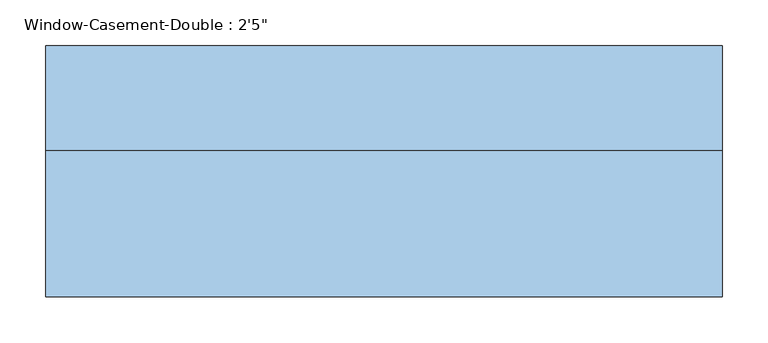
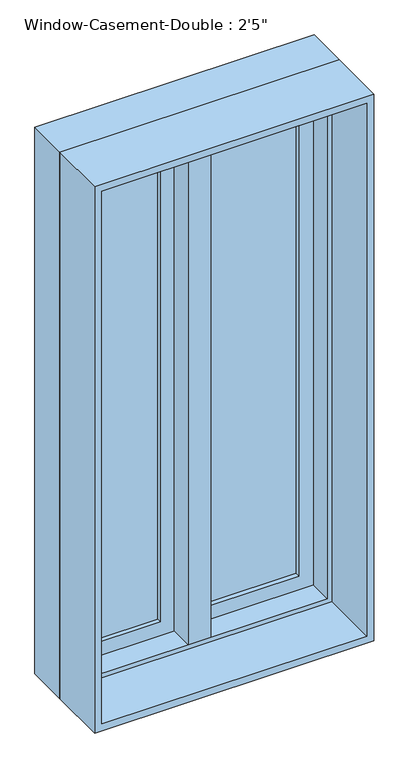
"""IFC4 building model written with IfcOpenShell, lengths in millimetres: window geometry."""

from ifc_helpers import new_model, si_unit, frame, origin, place, context, project, spatial, polyline, outline, extrude, faceted_brep, source, transform, mapped, element, save


def window_ba8015fa(model_context):
    return source(origin(), model_context, "Body", "SolidModel", [
        faceted_brep([(9.525, 146.05, 2425.7), (-9.525, 146.05, 2425.7), (-9.525, 95.25, 2425.7), (9.525, 95.25, 2425.7), (9.525, 146.05, 927.1), (9.525, 95.25, 927.1), (-9.525, 95.25, 927.1), (-9.525, 146.05, 927.1), (-9.525, 95.25, 946.15), (-9.525, 95.25, 2406.65), (-30.1625, 95.25, 946.15), (-30.1625, 95.25, 2406.65), (-30.1625, 31.75, 946.15), (-30.1625, 31.75, 2406.65), (30.1625, 31.75, 946.15), (30.1625, 31.75, 2406.65), (30.1625, 95.25, 946.15), (30.1625, 95.25, 2406.65), (9.525, 95.25, 946.15), (9.525, 95.25, 2406.65)], [[[0, 1, 2, 3]], [[4, 5, 6, 7]], [[1, 0, 4, 7]], [[2, 1, 7, 6, 8, 9]], [[9, 8, 10, 11]], [[11, 10, 12, 13]], [[13, 12, 14, 15]], [[15, 14, 16, 17]], [[17, 16, 18, 19]], [[0, 3, 19, 18, 5, 4]], [[18, 8, 6, 5]], [[9, 19, 3, 2]], [[8, 18, 16, 14, 12, 10]], [[19, 9, 11, 13, 15, 17]]]),
        extrude(outline(polyline([(-66.675, 127.0), (-66.675, 120.65), (-298.45, 120.65), (-298.45, 127.0), (-66.675, 127.0)])), frame((0.0, 0.0, 984.25), z_axis=(0.0, 0.0, 1.0), x_axis=(1.0, 0.0, 0.0)), (0.0, 0.0, 1.0), 1384.3),
        extrude(outline(polyline([(-298.45, 107.95), (-298.45, 114.3), (-66.675, 114.3), (-66.675, 107.95), (-298.45, 107.95)])), frame((0.0, 0.0, 984.25), z_axis=(0.0, 0.0, 1.0), x_axis=(1.0, 0.0, 0.0)), (0.0, 0.0, 1.0), 1384.3),
        extrude(outline(polyline([(298.45, 127.0), (298.45, 120.65), (66.675, 120.65), (66.675, 127.0), (298.45, 127.0)])), frame((0.0, 0.0, 984.25), z_axis=(0.0, 0.0, 1.0), x_axis=(1.0, 0.0, 0.0)), (0.0, 0.0, 1.0), 1384.3),
        extrude(outline(polyline([(66.675, 107.95), (66.675, 114.3), (298.45, 114.3), (298.45, 107.95), (66.675, 107.95)])), frame((0.0, 0.0, 984.25), z_axis=(0.0, 0.0, 1.0), x_axis=(1.0, 0.0, 0.0)), (0.0, 0.0, 1.0), 1384.3),
        extrude(outline(polyline([(2425.7, -355.6), (927.1, -355.6), (927.1, -9.525), (2425.7, -9.525), (2425.7, -355.6)]), holes=[polyline([(2368.55, -66.675), (984.25, -66.675), (984.25, -298.45), (2368.55, -298.45), (2368.55, -66.675)])]), frame((0.0, 95.25, 0.0), z_axis=(0.0, 1.0, 0.0), x_axis=(0.0, 0.0, 1.0)), (0.0, 0.0, 1.0), 44.45),
        extrude(outline(polyline([(927.1, 355.6), (2425.7, 355.6), (2425.7, 9.525), (927.1, 9.525), (927.1, 355.6)]), holes=[polyline([(984.25, 66.675), (2368.55, 66.675), (2368.55, 298.45), (984.25, 298.45), (984.25, 66.675)])]), frame((0.0, 95.25, 0.0), z_axis=(0.0, 1.0, 0.0), x_axis=(0.0, 0.0, 1.0)), (0.0, 0.0, 1.0), 44.45),
        extrude(outline(polyline([(2438.4, -368.3), (914.4, -368.3), (914.4, 368.3), (2438.4, 368.3), (2438.4, -368.3)]), holes=[polyline([(2419.35, 349.25), (933.45, 349.25), (933.45, -349.25), (2419.35, -349.25), (2419.35, 349.25)])]), frame((0.0, -127.0, 0.0), z_axis=(0.0, 1.0, 0.0), x_axis=(0.0, 0.0, 1.0)), (0.0, 0.0, 1.0), 158.75),
        faceted_brep([(336.55, 95.25, 2406.65), (336.55, 31.75, 2406.65), (-336.55, 31.75, 2406.65), (-336.55, 95.25, 2406.65), (355.6, 146.05, 2425.7), (355.6, 95.25, 2425.7), (-355.6, 95.25, 2425.7), (-355.6, 146.05, 2425.7), (368.3, 31.75, 2438.4), (368.3, 146.05, 2438.4), (-368.3, 146.05, 2438.4), (-368.3, 31.75, 2438.4), (-336.55, 31.75, 946.15), (-336.55, 95.25, 946.15), (-355.6, 95.25, 927.1), (-355.6, 146.05, 927.1), (-368.3, 146.05, 914.4), (-368.3, 31.75, 914.4), (336.55, 31.75, 946.15), (336.55, 95.25, 946.15), (355.6, 95.25, 927.1), (355.6, 146.05, 927.1), (368.3, 146.05, 914.4), (368.3, 31.75, 914.4)], [[[0, 1, 2, 3]], [[4, 5, 6, 7]], [[8, 9, 10, 11]], [[3, 2, 12, 13]], [[7, 6, 14, 15]], [[11, 10, 16, 17]], [[13, 12, 18, 19]], [[15, 14, 20, 21]], [[17, 16, 22, 23]], [[11, 17, 23, 8], [1, 18, 12, 2]], [[19, 18, 1, 0]], [[5, 20, 14, 6], [3, 13, 19, 0]], [[21, 20, 5, 4]], [[23, 22, 9, 8]], [[9, 22, 16, 10], [7, 15, 21, 4]]]),
    ])


if __name__ == "__main__":
    model = new_model("IFC4")
    model_context = context("Model", 3, world=origin())
    ifc_project = project(units=[si_unit("LENGTHUNIT", "METRE", prefix="MILLI")], contexts=[model_context])
    site = spatial("IfcSite", under=ifc_project)
    building = spatial("IfcBuilding", under=site)
    placement = place(None, origin())
    window_shape = window_ba8015fa(model_context)
    element("IfcWindow", 1, ObjectType="Window-Casement-Double : 2'5\"", at=placement, inside=building, context=model_context, shape_type="MappedRepresentation", body=[
        mapped(window_shape, transform((0.0, 0.0, 0.0), x_axis=(1.0, 0.0, 0.0), y_axis=(0.0, 1.0, 0.0), z_axis=(0.0, 0.0, 1.0))),
    ])
    save(model, "model.ifc")

# Revit data of these elements
# Type "Window-Casement-Double : 2'5\""
#   Type Mark = "19"
#   Fire Rating = "0.5h"
#   Assembly Code = "B2020100"
#   Analytic Construction = "Double glazing - domestic"
#   Frame Extension [instance default] = 0' - 0 1/4"
#   Window Inset [instance default] = 0' - 0"
#   Wall Thickness [instance default] = 0' - 6"
#   Interior Wall Closure [instance default] = 0' - 2 1/4"
#   Half Width = 1' - 2 1/2"
#   Visual Light Transmittance = 0.81
#   Thermal Resistance (R) = 1.8146 (h·ft²·°F)/BTU
#   Solar Heat Gain Coefficient = 0.76
#   Rough Width = 2' - 5 1/2"
#   Rough Height = 5' - 0 1/2"
#   Height = 5' - 0"
#   Heat Transfer Coefficient (U) = 0.5511 BTU/(h·ft²·°F)
#   Exterior Wall Closure [instance default] = 0' - 1 1/4"
#   Extension Jamb [instance default] = 0' - 2 1/4"
#   Default Sill Height = 3' - 0"
#   Width = 2' - 5"
#   Muntin Visibility = yes
#   Interior Trim Visibility [instance default] = yes
#   Exterior Trim Visibility [instance default] = yes
#   Extension Jamb Visibility [instance default] = yes
#   Interior Trim Material = Wood - Stained
#   Muntin Pattern = Muntin Pattern_2x2 : Muntin Pattern_2x2
#   Interior Trim = Trim-Window-Interior-Flat : Picture Frame
#   Interior Frame Material = Wood - Stained
#   Glass Panel Material = Glass
#   Exterior Trim Material = Clad - White
#   Exterior Trim = Trim-Window-Exterior-Flat : with Sill
#   Exterior Frame Material = Clad - White
#   Wall Closure = (empty or 0)
# Element 1 (IfcWindow, "Window-Casement-Double : 2'5\"")
#   Wall Thickness = 0' - 10"
#   Extension Jamb = 0' - 6 1/4"
#   Materials on its faces: "Wood - Stained", "Glass", "Clad - White"
# Materials
#   "Wood - Stained": class "Wood", colour RGB 224 178 126, transparency 0, Cost = 0
#   "Glass": class "Glass", colour RGB 0 128 192, transparency 0.75, Description = "Soda Lime Glass", Cost = 0
#   "Clad - White": class "Wood", colour RGB 242 242 238, transparency 0, Cost = 0
